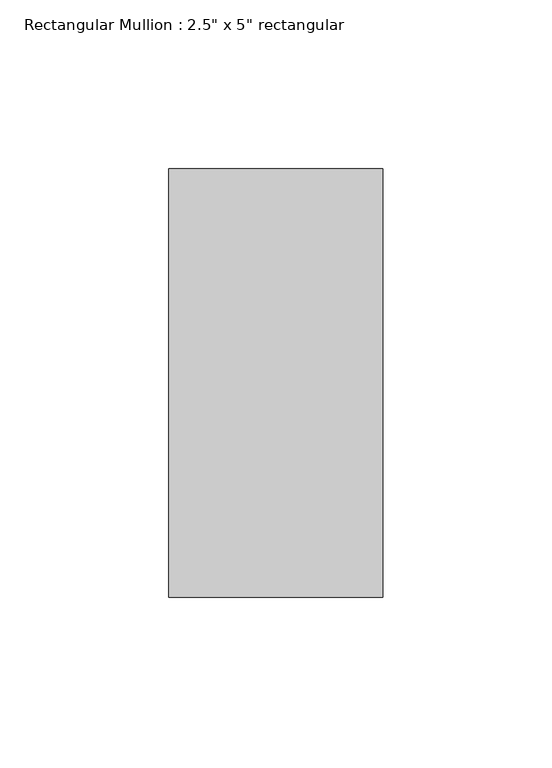
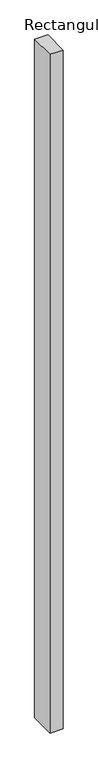
"""IFC4 building model written with IfcOpenShell, lengths in millimetres: member geometry."""

from ifc_helpers import new_model, si_unit, frame, origin, place, context, project, spatial, polyline, outline, extrude, source, transform, mapped, element, save


def member_fce16bad(model_context):
    return source(origin(), model_context, "Body", "SweptSolid", [
        extrude(outline(polyline([(0.0, 63.5), (0.0, -63.5), (-63.5, -63.5), (-63.5, 63.5), (0.0, 63.5)])), frame((0.0, 0.0, -3454.000116), z_axis=(0.0, 0.0, 1.0), x_axis=(1.0, 0.0, 0.0)), (0.0, 0.0, 1.0), 3454.000116),
    ])


if __name__ == "__main__":
    model = new_model("IFC4")
    model_context = context("Model", 3, world=origin())
    ifc_project = project(units=[si_unit("LENGTHUNIT", "METRE", prefix="MILLI")], contexts=[model_context])
    site = spatial("IfcSite", under=ifc_project)
    building = spatial("IfcBuilding", under=site)
    placement = place(None, origin())
    member_shape = member_fce16bad(model_context)
    element("IfcMember", 1, ObjectType="Rectangular Mullion : 2.5\" x 5\" rectangular", at=placement, inside=building, context=model_context, shape_type="MappedRepresentation", body=[
        mapped(member_shape, transform((0.0, 0.0, 0.0), x_axis=(1.0, 0.0, 0.0), y_axis=(0.0, 1.0, 0.0), z_axis=(0.0, 0.0, 1.0))),
    ])
    save(model, "model.ifc")

# Revit data of these elements
# Type "Rectangular Mullion : 2.5\" x 5\" rectangular"
#   built-in parameter 1007304 = 0.416667 (stored number, unit not read)
#   built-in parameter 1007301 = 0.104167 (stored number, unit not read)
#   built-in parameter 1007300 = 0.104167 (stored number, unit not read)
# Element 1 (IfcMember, "Rectangular Mullion : 2.5\" x 5\" rectangular")
#   Materials on its faces: "Aluminum"
# Materials
#   "Aluminum": class "Metal", colour RGB 247 247 247, transparency 0, Description = "Aluminum 6061", Cost = 0
